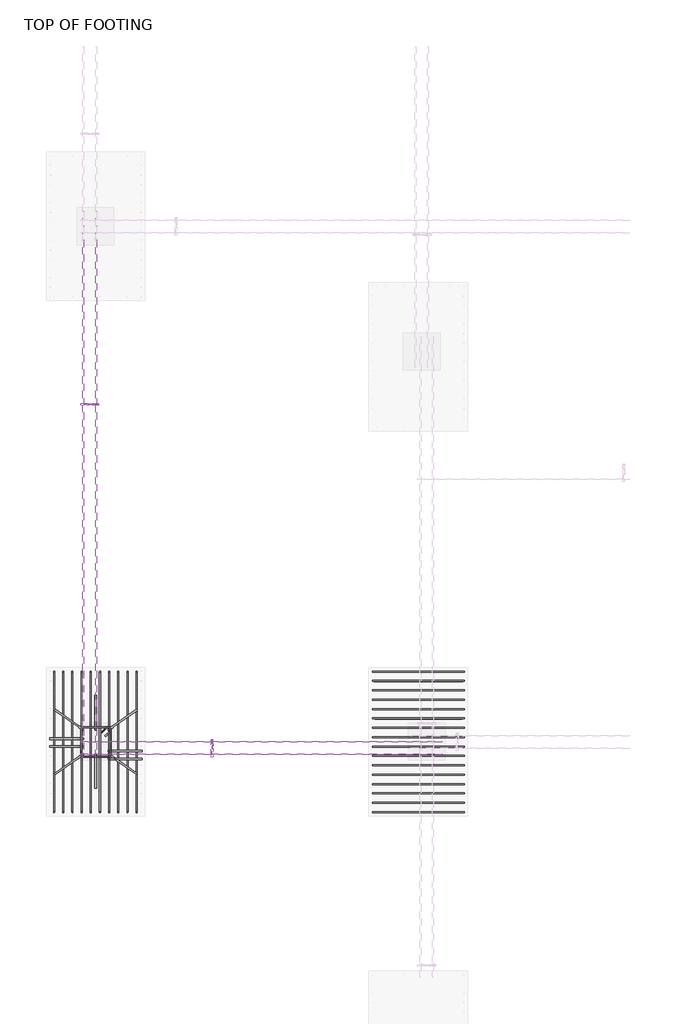
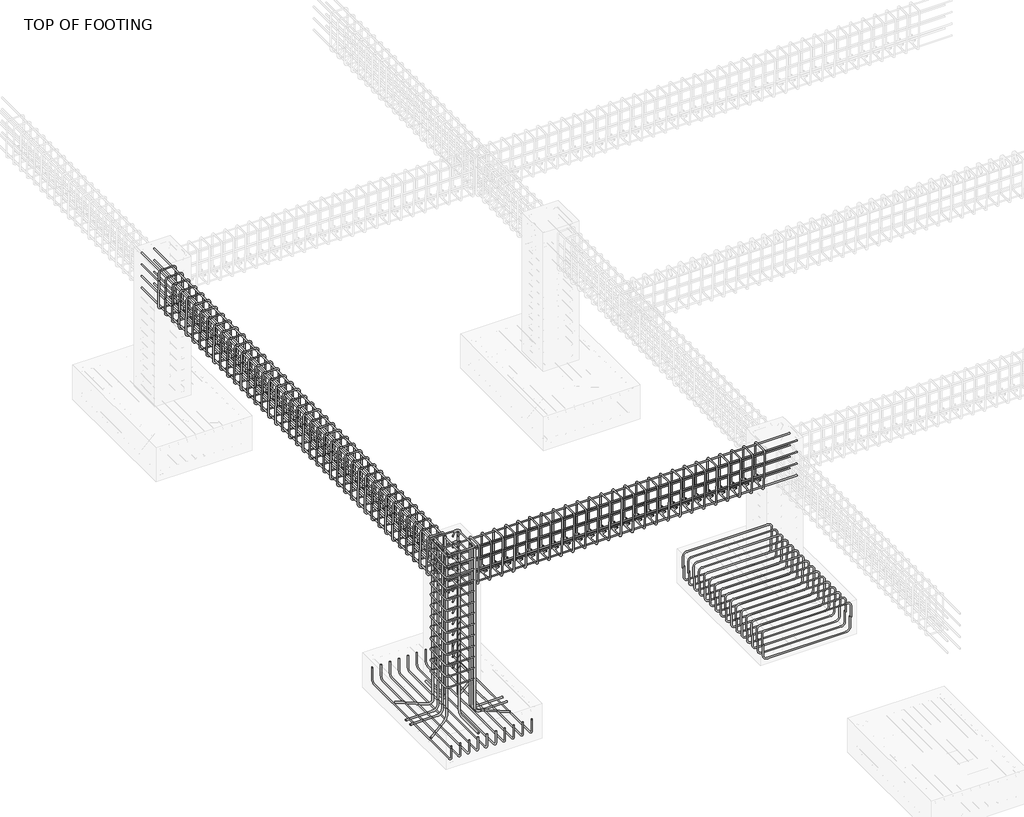
# One storey, part 3 of 11: 18 reinforcing bars.
"""IFC4 building model written with IfcOpenShell, lengths in millimetres."""

from ifc_helpers import new_model, si_unit, point, frame, origin, place, context, project, spatial, polyline, circle_curve, trimmed, segment, composite_curve, source, transform, mapped, element, save
from ifc_brep_helpers import swept_disk

model = new_model("IFC4")

# Units and contexts
model_context = context("Model", 3, world=origin())
ifc_project = project(units=[si_unit("LENGTHUNIT", "METRE", prefix="MILLI")], contexts=[model_context])

# Site, building, storey
site = spatial("IfcSite", under=ifc_project)
building = spatial("IfcBuilding", under=site)
storey = spatial("IfcBuildingStorey", under=building, Name="TOP OF FOOTING", Elevation=-1828.8)

# Reinforcing bars
placement = place(None, origin())
reinforcing_bar_shape = source(origin(), model_context, "Body", "SolidModel", [
    swept_disk(composite_curve([segment(polyline([(-6783.9053871, -2335.4013044, -2021.5298587), (-6783.9053871, -2335.4013044, -2168.8298587)]), True, "CONTINUOUS"), segment(trimmed(circle_curve(frame((-6783.9053871, -2381.7513044, -2168.8298587), z_axis=(-1.0, 0.0, 0.0), x_axis=(0.0, 46.350000000000364, 0.0)), 46.35), [point((-6783.9053871, -2335.4013044, -2168.8298587))], [point((-6783.9053871, -2381.7513044, -2215.1798587))], True, "CARTESIAN"), True, "CONTINUOUS"), segment(polyline([(-6783.9053871, -2381.7513044, -2215.1798587), (-6783.9053871, -3996.3513044, -2215.1798587)]), True, "CONTINUOUS"), segment(trimmed(circle_curve(frame((-6783.9053871, -3996.3513044, -2168.8298587), z_axis=(-1.0, 0.0, 0.0), x_axis=(0.0, 0.0, -46.34999999999991)), 46.35), [point((-6783.9053871, -3996.3513044, -2215.1798587))], [point((-6783.9053871, -4042.7013044, -2168.8298587))], True, "CARTESIAN"), True, "CONTINUOUS"), segment(polyline([(-6783.9053871, -4042.7013044, -2168.8298587), (-6783.9053871, -4042.7013044, -2021.5298587)]), True, "CONTINUOUS")], self_intersect=False), 6.35),
])
element("IfcReinforcingBar", 1, at=placement, inside=storey, context=model_context, shape_type="MappedRepresentation", body=[
    mapped(reinforcing_bar_shape, transform((0.0, 0.0, 0.0), x_axis=(1.0, 0.0, 0.0), y_axis=(0.0, 1.0, 0.0), z_axis=(0.0, 0.0, 1.0))),
    mapped(reinforcing_bar_shape, transform((111.55177, 0.0, 0.0), x_axis=(1.0, 0.0, 0.0), y_axis=(0.0, 1.0, 0.0), z_axis=(0.0, 0.0, 1.0))),
    mapped(reinforcing_bar_shape, transform((223.10354, 0.0, 0.0), x_axis=(1.0, 0.0, 0.0), y_axis=(0.0, 1.0, 0.0), z_axis=(0.0, 0.0, 1.0))),
    mapped(reinforcing_bar_shape, transform((334.6553099, 0.0, 0.0), x_axis=(1.0, 0.0, 0.0), y_axis=(0.0, 1.0, 0.0), z_axis=(0.0, 0.0, 1.0))),
    mapped(reinforcing_bar_shape, transform((446.2070799, 0.0, 0.0), x_axis=(1.0, 0.0, 0.0), y_axis=(0.0, 1.0, 0.0), z_axis=(0.0, 0.0, 1.0))),
    mapped(reinforcing_bar_shape, transform((557.7588499, 0.0, 0.0), x_axis=(1.0, 0.0, 0.0), y_axis=(0.0, 1.0, 0.0), z_axis=(0.0, 0.0, 1.0))),
    mapped(reinforcing_bar_shape, transform((669.3106199, 0.0, 0.0), x_axis=(1.0, 0.0, 0.0), y_axis=(0.0, 1.0, 0.0), z_axis=(0.0, 0.0, 1.0))),
    mapped(reinforcing_bar_shape, transform((780.8623899, 0.0, 0.0), x_axis=(1.0, 0.0, 0.0), y_axis=(0.0, 1.0, 0.0), z_axis=(0.0, 0.0, 1.0))),
    mapped(reinforcing_bar_shape, transform((892.4141599, 0.0, 0.0), x_axis=(1.0, 0.0, 0.0), y_axis=(0.0, 1.0, 0.0), z_axis=(0.0, 0.0, 1.0))),
    mapped(reinforcing_bar_shape, transform((1003.9659298, 0.0, 0.0), x_axis=(1.0, 0.0, 0.0), y_axis=(0.0, 1.0, 0.0), z_axis=(0.0, 0.0, 1.0))),
])
reinforcing_bar_2_shape = source(origin(), model_context, "Body", "SolidModel", [
    swept_disk(composite_curve([segment(polyline([(-1813.2210247, -2335.4013044, -2046.7466921), (-1813.2210247, -2335.4013044, -2194.0466921)]), True, "CONTINUOUS"), segment(trimmed(circle_curve(frame((-1859.5710247, -2335.4013044, -2194.0466921), z_axis=(0.0, 1.0, 0.0), x_axis=(46.34999999999991, 0.0, 0.0)), 46.35), [point((-1813.2210247, -2335.4013044, -2194.0466921))], [point((-1859.5710247, -2335.4013044, -2240.3966921))], True, "CARTESIAN"), True, "CONTINUOUS"), segment(polyline([(-1859.5710247, -2335.4013044, -2240.3966921), (-2850.7992774, -2335.4013044, -2240.3966921)]), True, "CONTINUOUS"), segment(trimmed(circle_curve(frame((-2850.7992774, -2335.4013044, -2194.0466921), z_axis=(0.0, 1.0, 0.0), x_axis=(0.0, 0.0, -46.34999999999991)), 46.35), [point((-2850.7992774, -2335.4013044, -2240.3966921))], [point((-2897.1492774, -2335.4013044, -2194.0466921))], True, "CARTESIAN"), True, "CONTINUOUS"), segment(polyline([(-2897.1492774, -2335.4013044, -2194.0466921), (-2897.1492774, -2335.4013044, -2046.7466921)]), True, "CONTINUOUS")], self_intersect=False), 6.35),
])
element("IfcReinforcingBar", 2, at=placement, inside=storey, context=model_context, shape_type="MappedRepresentation", body=[
    mapped(reinforcing_bar_2_shape, transform((0.0, 0.0, 0.0), x_axis=(1.0, 0.0, 0.0), y_axis=(0.0, 1.0, 0.0), z_axis=(0.0, 0.0, 1.0))),
    mapped(reinforcing_bar_2_shape, transform((0.0, -113.82, 0.0), x_axis=(1.0, 0.0, 0.0), y_axis=(0.0, 1.0, 0.0), z_axis=(0.0, 0.0, 1.0))),
    mapped(reinforcing_bar_2_shape, transform((0.0, -227.64, 0.0), x_axis=(1.0, 0.0, 0.0), y_axis=(0.0, 1.0, 0.0), z_axis=(0.0, 0.0, 1.0))),
    mapped(reinforcing_bar_2_shape, transform((0.0, -341.46, 0.0), x_axis=(1.0, 0.0, 0.0), y_axis=(0.0, 1.0, 0.0), z_axis=(0.0, 0.0, 1.0))),
    mapped(reinforcing_bar_2_shape, transform((0.0, -455.28, 0.0), x_axis=(1.0, 0.0, 0.0), y_axis=(0.0, 1.0, 0.0), z_axis=(0.0, 0.0, 1.0))),
    mapped(reinforcing_bar_2_shape, transform((0.0, -569.1, 0.0), x_axis=(1.0, 0.0, 0.0), y_axis=(0.0, 1.0, 0.0), z_axis=(0.0, 0.0, 1.0))),
    mapped(reinforcing_bar_2_shape, transform((0.0, -682.92, 0.0), x_axis=(1.0, 0.0, 0.0), y_axis=(0.0, 1.0, 0.0), z_axis=(0.0, 0.0, 1.0))),
    mapped(reinforcing_bar_2_shape, transform((0.0, -796.74, 0.0), x_axis=(1.0, 0.0, 0.0), y_axis=(0.0, 1.0, 0.0), z_axis=(0.0, 0.0, 1.0))),
    mapped(reinforcing_bar_2_shape, transform((0.0, -910.56, 0.0), x_axis=(1.0, 0.0, 0.0), y_axis=(0.0, 1.0, 0.0), z_axis=(0.0, 0.0, 1.0))),
    mapped(reinforcing_bar_2_shape, transform((0.0, -1024.38, 0.0), x_axis=(1.0, 0.0, 0.0), y_axis=(0.0, 1.0, 0.0), z_axis=(0.0, 0.0, 1.0))),
    mapped(reinforcing_bar_2_shape, transform((0.0, -1138.2, 0.0), x_axis=(1.0, 0.0, 0.0), y_axis=(0.0, 1.0, 0.0), z_axis=(0.0, 0.0, 1.0))),
    mapped(reinforcing_bar_2_shape, transform((0.0, -1252.02, 0.0), x_axis=(1.0, 0.0, 0.0), y_axis=(0.0, 1.0, 0.0), z_axis=(0.0, 0.0, 1.0))),
    mapped(reinforcing_bar_2_shape, transform((0.0, -1365.84, 0.0), x_axis=(1.0, 0.0, 0.0), y_axis=(0.0, 1.0, 0.0), z_axis=(0.0, 0.0, 1.0))),
    mapped(reinforcing_bar_2_shape, transform((0.0, -1479.66, 0.0), x_axis=(1.0, 0.0, 0.0), y_axis=(0.0, 1.0, 0.0), z_axis=(0.0, 0.0, 1.0))),
    mapped(reinforcing_bar_2_shape, transform((0.0, -1593.48, 0.0), x_axis=(1.0, 0.0, 0.0), y_axis=(0.0, 1.0, 0.0), z_axis=(0.0, 0.0, 1.0))),
    mapped(reinforcing_bar_2_shape, transform((0.0, -1707.3, 0.0), x_axis=(1.0, 0.0, 0.0), y_axis=(0.0, 1.0, 0.0), z_axis=(0.0, 0.0, 1.0))),
])
reinforcing_bar_3_shape = source(origin(), model_context, "Body", "SolidModel", [
    swept_disk(composite_curve([segment(polyline([(-2909.0228049, -2335.4013044, -2061.9958198), (-2909.0228049, -2335.4013044, -1914.6958198)]), True, "CONTINUOUS"), segment(trimmed(circle_curve(frame((-2862.6728049, -2335.4013044, -1914.6958198), z_axis=(0.0, 1.0, 0.0), x_axis=(-46.350000000000364, 0.0, 0.0)), 46.35), [point((-2909.0228049, -2335.4013044, -1914.6958198))], [point((-2862.6728049, -2335.4013044, -1868.3458198))], True, "CARTESIAN"), True, "CONTINUOUS"), segment(polyline([(-2862.6728049, -2335.4013044, -1868.3458198), (-1848.0728049, -2335.4013044, -1868.3458198)]), True, "CONTINUOUS"), segment(trimmed(circle_curve(frame((-1848.0728049, -2335.4013044, -1914.6958198), z_axis=(0.0, 1.0, 0.0), x_axis=(0.0, 0.0, 46.34999999999991)), 46.35), [point((-1848.0728049, -2335.4013044, -1868.3458198))], [point((-1801.7228049, -2335.4013044, -1914.6958198))], True, "CARTESIAN"), True, "CONTINUOUS"), segment(polyline([(-1801.7228049, -2335.4013044, -1914.6958198), (-1801.7228049, -2335.4013044, -2061.9958198)]), True, "CONTINUOUS")], self_intersect=False), 6.35),
])
element("IfcReinforcingBar", 3, at=placement, inside=storey, context=model_context, shape_type="MappedRepresentation", body=[
    mapped(reinforcing_bar_3_shape, transform((0.0, 0.0, 0.0), x_axis=(1.0, 0.0, 0.0), y_axis=(0.0, 1.0, 0.0), z_axis=(0.0, 0.0, 1.0))),
    mapped(reinforcing_bar_3_shape, transform((0.0, -113.82, 0.0), x_axis=(1.0, 0.0, 0.0), y_axis=(0.0, 1.0, 0.0), z_axis=(0.0, 0.0, 1.0))),
    mapped(reinforcing_bar_3_shape, transform((0.0, -227.64, 0.0), x_axis=(1.0, 0.0, 0.0), y_axis=(0.0, 1.0, 0.0), z_axis=(0.0, 0.0, 1.0))),
    mapped(reinforcing_bar_3_shape, transform((0.0, -341.46, 0.0), x_axis=(1.0, 0.0, 0.0), y_axis=(0.0, 1.0, 0.0), z_axis=(0.0, 0.0, 1.0))),
    mapped(reinforcing_bar_3_shape, transform((0.0, -455.28, 0.0), x_axis=(1.0, 0.0, 0.0), y_axis=(0.0, 1.0, 0.0), z_axis=(0.0, 0.0, 1.0))),
    mapped(reinforcing_bar_3_shape, transform((0.0, -569.1, 0.0), x_axis=(1.0, 0.0, 0.0), y_axis=(0.0, 1.0, 0.0), z_axis=(0.0, 0.0, 1.0))),
    mapped(reinforcing_bar_3_shape, transform((0.0, -682.92, 0.0), x_axis=(1.0, 0.0, 0.0), y_axis=(0.0, 1.0, 0.0), z_axis=(0.0, 0.0, 1.0))),
    mapped(reinforcing_bar_3_shape, transform((0.0, -796.74, 0.0), x_axis=(1.0, 0.0, 0.0), y_axis=(0.0, 1.0, 0.0), z_axis=(0.0, 0.0, 1.0))),
    mapped(reinforcing_bar_3_shape, transform((0.0, -910.56, 0.0), x_axis=(1.0, 0.0, 0.0), y_axis=(0.0, 1.0, 0.0), z_axis=(0.0, 0.0, 1.0))),
    mapped(reinforcing_bar_3_shape, transform((0.0, -1024.38, 0.0), x_axis=(1.0, 0.0, 0.0), y_axis=(0.0, 1.0, 0.0), z_axis=(0.0, 0.0, 1.0))),
    mapped(reinforcing_bar_3_shape, transform((0.0, -1138.2, 0.0), x_axis=(1.0, 0.0, 0.0), y_axis=(0.0, 1.0, 0.0), z_axis=(0.0, 0.0, 1.0))),
    mapped(reinforcing_bar_3_shape, transform((0.0, -1252.02, 0.0), x_axis=(1.0, 0.0, 0.0), y_axis=(0.0, 1.0, 0.0), z_axis=(0.0, 0.0, 1.0))),
    mapped(reinforcing_bar_3_shape, transform((0.0, -1365.84, 0.0), x_axis=(1.0, 0.0, 0.0), y_axis=(0.0, 1.0, 0.0), z_axis=(0.0, 0.0, 1.0))),
    mapped(reinforcing_bar_3_shape, transform((0.0, -1479.66, 0.0), x_axis=(1.0, 0.0, 0.0), y_axis=(0.0, 1.0, 0.0), z_axis=(0.0, 0.0, 1.0))),
    mapped(reinforcing_bar_3_shape, transform((0.0, -1593.48, 0.0), x_axis=(1.0, 0.0, 0.0), y_axis=(0.0, 1.0, 0.0), z_axis=(0.0, 0.0, 1.0))),
    mapped(reinforcing_bar_3_shape, transform((0.0, -1707.3, 0.0), x_axis=(1.0, 0.0, 0.0), y_axis=(0.0, 1.0, 0.0), z_axis=(0.0, 0.0, 1.0))),
])
reinforcing_bar_4_shape = source(origin(), model_context, "Body", "SolidModel", [
    swept_disk(composite_curve([segment(polyline([(-6205.9841654, -3075.3270697, -46.35), (-6150.2406025, -3019.5835068, -46.35)]), True, "CONTINUOUS"), segment(trimmed(circle_curve(frame((-6128.0728049, -3041.7513044, -46.35), z_axis=(0.0, 0.0, -1.0), x_axis=(-22.167797600000085, 22.167797600000085, 0.0)), 31.35), [point((-6150.2406025, -3019.5835068, -46.35))], [point((-6096.7228049, -3041.7513044, -46.35))], True, "CARTESIAN"), True, "CONTINUOUS"), segment(polyline([(-6096.7228049, -3041.7513044, -46.35), (-6096.7228049, -3336.3513044, -46.35)]), True, "CONTINUOUS"), segment(trimmed(circle_curve(frame((-6128.0728049, -3336.3513044, -46.35), z_axis=(0.0, 0.0, -1.0), x_axis=(31.350000000000364, 0.0, 0.0)), 31.35), [point((-6096.7228049, -3336.3513044, -46.35))], [point((-6128.0728049, -3367.7013044, -46.35))], True, "CARTESIAN"), True, "CONTINUOUS"), segment(polyline([(-6128.0728049, -3367.7013044, -46.35), (-6422.6728049, -3367.7013044, -46.35)]), True, "CONTINUOUS"), segment(trimmed(circle_curve(frame((-6422.6728049, -3336.3710895, -45.2363875), z_axis=(0.0, 0.0355219283344819, -0.9993688971583016), x_axis=(0.0, -31.3302149000001, -1.1136125000000021)), 31.35), [point((-6422.6728049, -3367.7013044, -46.35))], [point((-6454.0228049, -3336.3710895, -45.2363875))], True, "CARTESIAN"), True, "CONTINUOUS"), segment(polyline([(-6454.0228049, -3336.3710895, -45.2363875), (-6454.0228049, -3041.7315193, -34.7636125)]), True, "CONTINUOUS"), segment(trimmed(circle_curve(frame((-6422.6728049, -3041.7315193, -34.7636125), z_axis=(0.0, 0.0355219283344819, -0.9993688971583016), x_axis=(-31.349999999999454, 0.0, 0.0)), 31.35), [point((-6454.0228049, -3041.7315193, -34.7636125))], [point((-6422.6728049, -3010.4013044, -33.65))], True, "CARTESIAN"), True, "CONTINUOUS"), segment(polyline([(-6422.6728049, -3010.4013044, -33.65), (-6128.0728049, -3010.4013044, -33.65)]), True, "CONTINUOUS"), segment(trimmed(circle_curve(frame((-6128.0728049, -3041.7513044, -33.65), z_axis=(0.0, 0.0, -1.0), x_axis=(0.0, 31.350000000000364, 0.0)), 31.35), [point((-6128.0728049, -3010.4013044, -33.65))], [point((-6105.9050073, -3063.919102, -33.65))], True, "CARTESIAN"), True, "CONTINUOUS"), segment(polyline([(-6105.9050073, -3063.919102, -33.65), (-6161.6485703, -3119.6626649, -33.65)]), True, "CONTINUOUS")], self_intersect=False), 6.35),
])
element("IfcReinforcingBar", 4, at=placement, inside=storey, context=model_context, shape_type="MappedRepresentation", body=[
    mapped(reinforcing_bar_4_shape, transform((0.0, 0.0, 0.0), x_axis=(1.0, 0.0, 0.0), y_axis=(0.0, 1.0, 0.0), z_axis=(0.0, 0.0, 1.0))),
    mapped(reinforcing_bar_4_shape, transform((0.0, 0.0, -144.675), x_axis=(1.0, 0.0, 0.0), y_axis=(0.0, 1.0, 0.0), z_axis=(0.0, 0.0, 1.0))),
    mapped(reinforcing_bar_4_shape, transform((0.0, 0.0, -289.35), x_axis=(1.0, 0.0, 0.0), y_axis=(0.0, 1.0, 0.0), z_axis=(0.0, 0.0, 1.0))),
    mapped(reinforcing_bar_4_shape, transform((0.0, 0.0, -434.025), x_axis=(1.0, 0.0, 0.0), y_axis=(0.0, 1.0, 0.0), z_axis=(0.0, 0.0, 1.0))),
    mapped(reinforcing_bar_4_shape, transform((0.0, 0.0, -578.7), x_axis=(1.0, 0.0, 0.0), y_axis=(0.0, 1.0, 0.0), z_axis=(0.0, 0.0, 1.0))),
    mapped(reinforcing_bar_4_shape, transform((0.0, 0.0, -723.375), x_axis=(1.0, 0.0, 0.0), y_axis=(0.0, 1.0, 0.0), z_axis=(0.0, 0.0, 1.0))),
    mapped(reinforcing_bar_4_shape, transform((0.0, 0.0, -868.05), x_axis=(1.0, 0.0, 0.0), y_axis=(0.0, 1.0, 0.0), z_axis=(0.0, 0.0, 1.0))),
    mapped(reinforcing_bar_4_shape, transform((0.0, 0.0, -1012.725), x_axis=(1.0, 0.0, 0.0), y_axis=(0.0, 1.0, 0.0), z_axis=(0.0, 0.0, 1.0))),
    mapped(reinforcing_bar_4_shape, transform((0.0, 0.0, -1157.4), x_axis=(1.0, 0.0, 0.0), y_axis=(0.0, 1.0, 0.0), z_axis=(0.0, 0.0, 1.0))),
    mapped(reinforcing_bar_4_shape, transform((0.0, 0.0, -1302.075), x_axis=(1.0, 0.0, 0.0), y_axis=(0.0, 1.0, 0.0), z_axis=(0.0, 0.0, 1.0))),
    mapped(reinforcing_bar_4_shape, transform((0.0, 0.0, -1446.75), x_axis=(1.0, 0.0, 0.0), y_axis=(0.0, 1.0, 0.0), z_axis=(0.0, 0.0, 1.0))),
    mapped(reinforcing_bar_4_shape, transform((0.0, 0.0, -1591.425), x_axis=(1.0, 0.0, 0.0), y_axis=(0.0, 1.0, 0.0), z_axis=(0.0, 0.0, 1.0))),
    mapped(reinforcing_bar_4_shape, transform((0.0, 0.0, -1736.1), x_axis=(1.0, 0.0, 0.0), y_axis=(0.0, 1.0, 0.0), z_axis=(0.0, 0.0, 1.0))),
])
reinforcing_bar_5_shape = source(origin(), model_context, "Body", "SolidModel", [
    swept_disk(composite_curve([segment(polyline([(-6118.0728049, -3300.4586931, -40.0), (-6118.0728049, -3300.4586931, -2136.75)]), True, "CONTINUOUS"), segment(trimmed(circle_curve(frame((-6051.0228049, -3300.4586931, -2136.75), z_axis=(0.0, -1.0, 0.0), x_axis=(-67.05000000000018, 0.0, 0.0)), 67.05), [point((-6118.0728049, -3300.4586931, -2136.75))], [point((-6051.0228049, -3300.4586931, -2203.8))], True, "CARTESIAN"), True, "CONTINUOUS"), segment(polyline([(-6051.0228049, -3300.4586931, -2203.8), (-5715.3728049, -3300.4586931, -2203.8)]), True, "CONTINUOUS")], self_intersect=False), 9.55),
])
element("IfcReinforcingBar", 5, at=placement, inside=storey, context=model_context, shape_type="MappedRepresentation", body=[
    mapped(reinforcing_bar_5_shape, transform((0.0, 0.0, 0.0), x_axis=(1.0, 0.0, 0.0), y_axis=(0.0, 1.0, 0.0), z_axis=(0.0, 0.0, 1.0))),
    mapped(reinforcing_bar_5_shape, transform((0.0, -94.3634327, 0.0), x_axis=(1.0, 0.0, 0.0), y_axis=(0.0, 1.0, 0.0), z_axis=(0.0, 0.0, 1.0))),
])
element("IfcReinforcingBar", 6, at=placement, inside=storey, context=model_context, shape_type="SolidModel", body=[
    swept_disk(composite_curve([segment(polyline([(-6118.0728049, -3340.0013044, -40.0), (-6118.0728049, -3340.0013044, -2136.75)]), True, "CONTINUOUS"), segment(trimmed(circle_curve(frame((-6063.1486603, -3378.4596044, -2136.75), z_axis=(-0.5735764363510477, -0.8191520442889907, 0.0), x_axis=(-54.924144599999636, 38.45829999999978, 0.0)), 67.05), [point((-6118.0728049, -3340.0013044, -2136.75))], [point((-6063.1486603, -3378.4596044, -2203.8))], True, "CARTESIAN"), True, "CONTINUOUS"), segment(polyline([(-6063.1486603, -3378.4596044, -2203.8), (-5780.0087562, -3576.7162997, -2203.8)]), True, "CONTINUOUS")], self_intersect=False), 9.55),
])
element("IfcReinforcingBar", 7, at=placement, inside=storey, context=model_context, shape_type="SolidModel", body=[
    swept_disk(composite_curve([segment(polyline([(-6118.0728049, -3038.1013044, -40.0), (-6118.0728049, -3038.1013044, -2136.75)]), True, "CONTINUOUS"), segment(trimmed(circle_curve(frame((-6063.1486603, -2999.6430043, -2136.75), z_axis=(0.5735764363510477, -0.8191520442889908, 0.0), x_axis=(-54.924144599999636, -38.45830010000009, 0.0)), 67.05), [point((-6118.0728049, -3038.1013044, -2136.75))], [point((-6063.1486603, -2999.6430043, -2203.8))], True, "CARTESIAN"), True, "CONTINUOUS"), segment(polyline([(-6063.1486603, -2999.6430043, -2203.8), (-5780.0087562, -2801.3863091, -2203.8)]), True, "CONTINUOUS")], self_intersect=False), 9.55),
])
element("IfcReinforcingBar", 8, at=placement, inside=storey, context=model_context, shape_type="SolidModel", body=[
    swept_disk(composite_curve([segment(polyline([(-6432.6728049, -3340.0013044, -40.0), (-6432.6728049, -3340.0013044, -2136.75)]), True, "CONTINUOUS"), segment(trimmed(circle_curve(frame((-6487.5969495, -3378.4596044, -2136.75), z_axis=(-0.5735764363510477, 0.8191520442889908, 0.0), x_axis=(54.924144599999636, 38.45829999999978, 0.0)), 67.05), [point((-6432.6728049, -3340.0013044, -2136.75))], [point((-6487.5969495, -3378.4596044, -2203.8))], True, "CARTESIAN"), True, "CONTINUOUS"), segment(polyline([(-6487.5969495, -3378.4596044, -2203.8), (-6770.7368536, -3576.7162997, -2203.8)]), True, "CONTINUOUS")], self_intersect=False), 9.55),
])
element("IfcReinforcingBar", 9, at=placement, inside=storey, context=model_context, shape_type="SolidModel", body=[
    swept_disk(composite_curve([segment(polyline([(-6432.6728049, -3038.1013044, -40.0), (-6432.6728049, -3038.1013044, -2136.75)]), True, "CONTINUOUS"), segment(trimmed(circle_curve(frame((-6487.5969495, -2999.6430043, -2136.75), z_axis=(0.5735764363510477, 0.8191520442889907, 0.0), x_axis=(54.924144599999636, -38.45830010000009, 0.0)), 67.05), [point((-6432.6728049, -3038.1013044, -2136.75))], [point((-6487.5969495, -2999.6430043, -2203.8))], True, "CARTESIAN"), True, "CONTINUOUS"), segment(polyline([(-6487.5969495, -2999.6430043, -2203.8), (-6770.7368536, -2801.3863091, -2203.8)]), True, "CONTINUOUS")], self_intersect=False), 9.55),
])
reinforcing_bar_6_shape = source(origin(), model_context, "Body", "SolidModel", [
    swept_disk(composite_curve([segment(polyline([(-6432.6728049, -3150.4586931, -40.0), (-6432.6728049, -3150.4586931, -2136.75)]), True, "CONTINUOUS"), segment(trimmed(circle_curve(frame((-6499.7228049, -3150.4586931, -2136.75), z_axis=(0.0, 1.0, 0.0), x_axis=(67.04999999999927, 0.0, 0.0)), 67.05), [point((-6432.6728049, -3150.4586931, -2136.75))], [point((-6499.7228049, -3150.4586931, -2203.8))], True, "CARTESIAN"), True, "CONTINUOUS"), segment(polyline([(-6499.7228049, -3150.4586931, -2203.8), (-6835.3728049, -3150.4586931, -2203.8)]), True, "CONTINUOUS")], self_intersect=False), 9.55),
])
element("IfcReinforcingBar", 10, at=placement, inside=storey, context=model_context, shape_type="MappedRepresentation", body=[
    mapped(reinforcing_bar_6_shape, transform((0.0, 0.0, 0.0), x_axis=(1.0, 0.0, 0.0), y_axis=(0.0, 1.0, 0.0), z_axis=(0.0, 0.0, 1.0))),
    mapped(reinforcing_bar_6_shape, transform((0.0, -94.3634327, 0.0), x_axis=(1.0, 0.0, 0.0), y_axis=(0.0, 1.0, 0.0), z_axis=(0.0, 0.0, 1.0))),
])
element("IfcReinforcingBar", 11, at=placement, inside=storey, context=model_context, shape_type="SolidModel", body=[
    swept_disk(composite_curve([segment(polyline([(-6278.0728049, -3038.1013044, -40.0), (-6278.0728049, -3038.1013044, -2136.75)]), True, "CONTINUOUS"), segment(trimmed(circle_curve(frame((-6278.0728049, -2971.0513044, -2136.75), z_axis=(1.0, 0.0, 0.0), x_axis=(0.0, -67.05000000000018, 0.0)), 67.05), [point((-6278.0728049, -3038.1013044, -2136.75))], [point((-6278.0728049, -2971.0513044, -2203.8))], True, "CARTESIAN"), True, "CONTINUOUS"), segment(polyline([(-6278.0728049, -2971.0513044, -2203.8), (-6278.0728049, -2625.4013044, -2203.8)]), True, "CONTINUOUS")], self_intersect=False), 9.55),
])
element("IfcReinforcingBar", 12, at=placement, inside=storey, context=model_context, shape_type="SolidModel", body=[
    swept_disk(composite_curve([segment(polyline([(-6278.0728049, -3340.0013044, -40.0), (-6278.0728049, -3340.0013044, -2136.75)]), True, "CONTINUOUS"), segment(trimmed(circle_curve(frame((-6278.0728049, -3407.0513044, -2136.75), z_axis=(-1.0, 0.0, 0.0), x_axis=(0.0, 67.04999999999973, 0.0)), 67.05), [point((-6278.0728049, -3340.0013044, -2136.75))], [point((-6278.0728049, -3407.0513044, -2203.8))], True, "CARTESIAN"), True, "CONTINUOUS"), segment(polyline([(-6278.0728049, -3407.0513044, -2203.8), (-6278.0728049, -3752.7013044, -2203.8)]), True, "CONTINUOUS")], self_intersect=False), 9.55),
])
reinforcing_bar_7_shape = source(origin(), model_context, "Body", "SolidModel", [
    swept_disk(composite_curve([segment(polyline([(-6355.9841654, 2837.5044674, -488.7242346), (-6300.2406025, 2837.5044674, -544.4677976)]), True, "CONTINUOUS"), segment(trimmed(circle_curve(frame((-6278.0728049, 2837.5044674, -522.3), z_axis=(0.0, -1.0, 0.0), x_axis=(-22.167797600000085, 0.0, -22.167797600000085)), 31.35), [point((-6300.2406025, 2837.5044674, -544.4677976))], [point((-6246.7228049, 2837.5044674, -522.3))], True, "CARTESIAN"), True, "CONTINUOUS"), segment(polyline([(-6246.7228049, 2837.5044674, -522.3), (-6246.7228049, 2837.5044674, -77.7)]), True, "CONTINUOUS"), segment(trimmed(circle_curve(frame((-6278.0728049, 2837.5044674, -77.7), z_axis=(0.0, -1.0, 0.0), x_axis=(31.350000000000364, 0.0, 0.0)), 31.35), [point((-6246.7228049, 2837.5044674, -77.7))], [point((-6278.0728049, 2837.5044674, -46.35))], True, "CARTESIAN"), True, "CONTINUOUS"), segment(polyline([(-6278.0728049, 2837.5044674, -46.35), (-6422.6728049, 2837.5044674, -46.35)]), True, "CONTINUOUS"), segment(trimmed(circle_curve(frame((-6422.6728049, 2838.289053, -77.6901807), z_axis=(0.0, -0.9996867842138424, -0.025026655153786322), x_axis=(0.0, -0.7845855999999003, 31.340180699999998)), 31.35), [point((-6422.6728049, 2837.5044674, -46.35))], [point((-6454.0228049, 2838.289053, -77.6901807))], True, "CARTESIAN"), True, "CONTINUOUS"), segment(polyline([(-6454.0228049, 2838.289053, -77.6901807), (-6454.0228049, 2849.4198817, -522.3098193)]), True, "CONTINUOUS"), segment(trimmed(circle_curve(frame((-6422.6728049, 2849.4198817, -522.3098193), z_axis=(0.0, -0.9996867842138424, -0.025026655153786322), x_axis=(-31.349999999999454, 0.0, 0.0)), 31.35), [point((-6454.0228049, 2849.4198817, -522.3098193))], [point((-6422.6728049, 2850.2044674, -553.65))], True, "CARTESIAN"), True, "CONTINUOUS"), segment(polyline([(-6422.6728049, 2850.2044674, -553.65), (-6278.0728049, 2850.2044674, -553.65)]), True, "CONTINUOUS"), segment(trimmed(circle_curve(frame((-6278.0728049, 2850.2044674, -522.3), z_axis=(0.0, -1.0, 0.0), x_axis=(0.0, 0.0, -31.350000000000023)), 31.35), [point((-6278.0728049, 2850.2044674, -553.65))], [point((-6255.9050073, 2850.2044674, -500.1322024))], True, "CARTESIAN"), True, "CONTINUOUS"), segment(polyline([(-6255.9050073, 2850.2044674, -500.1322024), (-6311.6485703, 2850.2044674, -444.3886395)]), True, "CONTINUOUS")], self_intersect=False), 6.35),
])
element("IfcReinforcingBar", 13, at=placement, inside=storey, context=model_context, shape_type="MappedRepresentation", body=[
    mapped(reinforcing_bar_7_shape, transform((0.0, 0.0, 0.0), x_axis=(1.0, 0.0, 0.0), y_axis=(0.0, 1.0, 0.0), z_axis=(0.0, 0.0, 1.0))),
    mapped(reinforcing_bar_7_shape, transform((0.0, -148.5950198, 0.0), x_axis=(1.0, 0.0, 0.0), y_axis=(0.0, 1.0, 0.0), z_axis=(0.0, 0.0, 1.0))),
    mapped(reinforcing_bar_7_shape, transform((0.0, -297.1900396, 0.0), x_axis=(1.0, 0.0, 0.0), y_axis=(0.0, 1.0, 0.0), z_axis=(0.0, 0.0, 1.0))),
    mapped(reinforcing_bar_7_shape, transform((0.0, -445.7850594, 0.0), x_axis=(1.0, 0.0, 0.0), y_axis=(0.0, 1.0, 0.0), z_axis=(0.0, 0.0, 1.0))),
    mapped(reinforcing_bar_7_shape, transform((0.0, -594.3800792, 0.0), x_axis=(1.0, 0.0, 0.0), y_axis=(0.0, 1.0, 0.0), z_axis=(0.0, 0.0, 1.0))),
    mapped(reinforcing_bar_7_shape, transform((0.0, -742.9750989, 0.0), x_axis=(1.0, 0.0, 0.0), y_axis=(0.0, 1.0, 0.0), z_axis=(0.0, 0.0, 1.0))),
    mapped(reinforcing_bar_7_shape, transform((0.0, -891.5701187, 0.0), x_axis=(1.0, 0.0, 0.0), y_axis=(0.0, 1.0, 0.0), z_axis=(0.0, 0.0, 1.0))),
    mapped(reinforcing_bar_7_shape, transform((0.0, -1040.1651385, 0.0), x_axis=(1.0, 0.0, 0.0), y_axis=(0.0, 1.0, 0.0), z_axis=(0.0, 0.0, 1.0))),
    mapped(reinforcing_bar_7_shape, transform((0.0, -1188.7601583, 0.0), x_axis=(1.0, 0.0, 0.0), y_axis=(0.0, 1.0, 0.0), z_axis=(0.0, 0.0, 1.0))),
    mapped(reinforcing_bar_7_shape, transform((0.0, -1337.3551781, 0.0), x_axis=(1.0, 0.0, 0.0), y_axis=(0.0, 1.0, 0.0), z_axis=(0.0, 0.0, 1.0))),
    mapped(reinforcing_bar_7_shape, transform((0.0, -1485.9501979, 0.0), x_axis=(1.0, 0.0, 0.0), y_axis=(0.0, 1.0, 0.0), z_axis=(0.0, 0.0, 1.0))),
    mapped(reinforcing_bar_7_shape, transform((0.0, -1634.5452177, 0.0), x_axis=(1.0, 0.0, 0.0), y_axis=(0.0, 1.0, 0.0), z_axis=(0.0, 0.0, 1.0))),
    mapped(reinforcing_bar_7_shape, transform((0.0, -1783.1402375, 0.0), x_axis=(1.0, 0.0, 0.0), y_axis=(0.0, 1.0, 0.0), z_axis=(0.0, 0.0, 1.0))),
    mapped(reinforcing_bar_7_shape, transform((0.0, -1931.7352573, 0.0), x_axis=(1.0, 0.0, 0.0), y_axis=(0.0, 1.0, 0.0), z_axis=(0.0, 0.0, 1.0))),
    mapped(reinforcing_bar_7_shape, transform((0.0, -2080.330277, 0.0), x_axis=(1.0, 0.0, 0.0), y_axis=(0.0, 1.0, 0.0), z_axis=(0.0, 0.0, 1.0))),
    mapped(reinforcing_bar_7_shape, transform((0.0, -2228.9252968, 0.0), x_axis=(1.0, 0.0, 0.0), y_axis=(0.0, 1.0, 0.0), z_axis=(0.0, 0.0, 1.0))),
    mapped(reinforcing_bar_7_shape, transform((0.0, -2377.5203166, 0.0), x_axis=(1.0, 0.0, 0.0), y_axis=(0.0, 1.0, 0.0), z_axis=(0.0, 0.0, 1.0))),
    mapped(reinforcing_bar_7_shape, transform((0.0, -2526.1153364, 0.0), x_axis=(1.0, 0.0, 0.0), y_axis=(0.0, 1.0, 0.0), z_axis=(0.0, 0.0, 1.0))),
    mapped(reinforcing_bar_7_shape, transform((0.0, -2674.7103562, 0.0), x_axis=(1.0, 0.0, 0.0), y_axis=(0.0, 1.0, 0.0), z_axis=(0.0, 0.0, 1.0))),
    mapped(reinforcing_bar_7_shape, transform((0.0, -2823.305376, 0.0), x_axis=(1.0, 0.0, 0.0), y_axis=(0.0, 1.0, 0.0), z_axis=(0.0, 0.0, 1.0))),
    mapped(reinforcing_bar_7_shape, transform((0.0, -2971.9003958, 0.0), x_axis=(1.0, 0.0, 0.0), y_axis=(0.0, 1.0, 0.0), z_axis=(0.0, 0.0, 1.0))),
    mapped(reinforcing_bar_7_shape, transform((0.0, -3120.4954156, 0.0), x_axis=(1.0, 0.0, 0.0), y_axis=(0.0, 1.0, 0.0), z_axis=(0.0, 0.0, 1.0))),
    mapped(reinforcing_bar_7_shape, transform((0.0, -3269.0904354, 0.0), x_axis=(1.0, 0.0, 0.0), y_axis=(0.0, 1.0, 0.0), z_axis=(0.0, 0.0, 1.0))),
    mapped(reinforcing_bar_7_shape, transform((0.0, -3417.6854551, 0.0), x_axis=(1.0, 0.0, 0.0), y_axis=(0.0, 1.0, 0.0), z_axis=(0.0, 0.0, 1.0))),
    mapped(reinforcing_bar_7_shape, transform((0.0, -3566.2804749, 0.0), x_axis=(1.0, 0.0, 0.0), y_axis=(0.0, 1.0, 0.0), z_axis=(0.0, 0.0, 1.0))),
    mapped(reinforcing_bar_7_shape, transform((0.0, -3714.8754947, 0.0), x_axis=(1.0, 0.0, 0.0), y_axis=(0.0, 1.0, 0.0), z_axis=(0.0, 0.0, 1.0))),
    mapped(reinforcing_bar_7_shape, transform((0.0, -3863.4705145, 0.0), x_axis=(1.0, 0.0, 0.0), y_axis=(0.0, 1.0, 0.0), z_axis=(0.0, 0.0, 1.0))),
    mapped(reinforcing_bar_7_shape, transform((0.0, -4012.0655343, 0.0), x_axis=(1.0, 0.0, 0.0), y_axis=(0.0, 1.0, 0.0), z_axis=(0.0, 0.0, 1.0))),
    mapped(reinforcing_bar_7_shape, transform((0.0, -4160.6605541, 0.0), x_axis=(1.0, 0.0, 0.0), y_axis=(0.0, 1.0, 0.0), z_axis=(0.0, 0.0, 1.0))),
    mapped(reinforcing_bar_7_shape, transform((0.0, -4309.2555739, 0.0), x_axis=(1.0, 0.0, 0.0), y_axis=(0.0, 1.0, 0.0), z_axis=(0.0, 0.0, 1.0))),
    mapped(reinforcing_bar_7_shape, transform((0.0, -4457.8505937, 0.0), x_axis=(1.0, 0.0, 0.0), y_axis=(0.0, 1.0, 0.0), z_axis=(0.0, 0.0, 1.0))),
    mapped(reinforcing_bar_7_shape, transform((0.0, -4606.4456135, 0.0), x_axis=(1.0, 0.0, 0.0), y_axis=(0.0, 1.0, 0.0), z_axis=(0.0, 0.0, 1.0))),
    mapped(reinforcing_bar_7_shape, transform((0.0, -4755.0406332, 0.0), x_axis=(1.0, 0.0, 0.0), y_axis=(0.0, 1.0, 0.0), z_axis=(0.0, 0.0, 1.0))),
    mapped(reinforcing_bar_7_shape, transform((0.0, -4903.635653, 0.0), x_axis=(1.0, 0.0, 0.0), y_axis=(0.0, 1.0, 0.0), z_axis=(0.0, 0.0, 1.0))),
    mapped(reinforcing_bar_7_shape, transform((0.0, -5052.2306728, 0.0), x_axis=(1.0, 0.0, 0.0), y_axis=(0.0, 1.0, 0.0), z_axis=(0.0, 0.0, 1.0))),
    mapped(reinforcing_bar_7_shape, transform((0.0, -5200.8256926, 0.0), x_axis=(1.0, 0.0, 0.0), y_axis=(0.0, 1.0, 0.0), z_axis=(0.0, 0.0, 1.0))),
    mapped(reinforcing_bar_7_shape, transform((0.0, -5349.4207124, 0.0), x_axis=(1.0, 0.0, 0.0), y_axis=(0.0, 1.0, 0.0), z_axis=(0.0, 0.0, 1.0))),
    mapped(reinforcing_bar_7_shape, transform((0.0, -5498.0157322, 0.0), x_axis=(1.0, 0.0, 0.0), y_axis=(0.0, 1.0, 0.0), z_axis=(0.0, 0.0, 1.0))),
    mapped(reinforcing_bar_7_shape, transform((0.0, -5646.610752, 0.0), x_axis=(1.0, 0.0, 0.0), y_axis=(0.0, 1.0, 0.0), z_axis=(0.0, 0.0, 1.0))),
    mapped(reinforcing_bar_7_shape, transform((0.0, -5795.2057718, 0.0), x_axis=(1.0, 0.0, 0.0), y_axis=(0.0, 1.0, 0.0), z_axis=(0.0, 0.0, 1.0))),
])
reinforcing_bar_8_shape = source(origin(), model_context, "Body", "SolidModel", [
    swept_disk(composite_curve([segment(polyline([(-6273.0728049, 3253.8544674, -528.2977114), (-6273.0728049, -3374.0513044, -528.2977114)]), True, "CONTINUOUS")], self_intersect=False), 6.35),
])
element("IfcReinforcingBar", 14, at=placement, inside=storey, context=model_context, shape_type="MappedRepresentation", body=[
    mapped(reinforcing_bar_8_shape, transform((0.0, 0.0, 0.0), x_axis=(1.0, 0.0, 0.0), y_axis=(0.0, 1.0, 0.0), z_axis=(0.0, 0.0, 1.0))),
    mapped(reinforcing_bar_8_shape, transform((0.0, 0.0, 153.3723948), x_axis=(1.0, 0.0, 0.0), y_axis=(0.0, 1.0, 0.0), z_axis=(0.0, 0.0, 1.0))),
    mapped(reinforcing_bar_8_shape, transform((0.0, 0.0, 306.7447895), x_axis=(1.0, 0.0, 0.0), y_axis=(0.0, 1.0, 0.0), z_axis=(0.0, 0.0, 1.0))),
    mapped(reinforcing_bar_8_shape, transform((0.0, 0.0, 460.1171843), x_axis=(1.0, 0.0, 0.0), y_axis=(0.0, 1.0, 0.0), z_axis=(0.0, 0.0, 1.0))),
])
reinforcing_bar_9_shape = source(origin(), model_context, "Body", "SolidModel", [
    swept_disk(composite_curve([segment(polyline([(-6427.6728049, 3253.8544674, -528.2977114), (-6427.6728049, -3374.0513044, -528.2977114)]), True, "CONTINUOUS")], self_intersect=False), 6.35),
])
element("IfcReinforcingBar", 15, at=placement, inside=storey, context=model_context, shape_type="MappedRepresentation", body=[
    mapped(reinforcing_bar_9_shape, transform((0.0, 0.0, 0.0), x_axis=(1.0, 0.0, 0.0), y_axis=(0.0, 1.0, 0.0), z_axis=(0.0, 0.0, 1.0))),
    mapped(reinforcing_bar_9_shape, transform((0.0, 0.0, 153.3723948), x_axis=(1.0, 0.0, 0.0), y_axis=(0.0, 1.0, 0.0), z_axis=(0.0, 0.0, 1.0))),
    mapped(reinforcing_bar_9_shape, transform((0.0, 0.0, 306.7447895), x_axis=(1.0, 0.0, 0.0), y_axis=(0.0, 1.0, 0.0), z_axis=(0.0, 0.0, 1.0))),
    mapped(reinforcing_bar_9_shape, transform((0.0, 0.0, 460.1171843), x_axis=(1.0, 0.0, 0.0), y_axis=(0.0, 1.0, 0.0), z_axis=(0.0, 0.0, 1.0))),
])
reinforcing_bar_10_shape = source(origin(), model_context, "Body", "SolidModel", [
    swept_disk(composite_curve([segment(polyline([(-6044.0228049, -3269.6626649, -488.7242346), (-6044.0228049, -3213.919102, -544.4677976)]), True, "CONTINUOUS"), segment(trimmed(circle_curve(frame((-6044.0228049, -3191.7513044, -522.3), z_axis=(1.0, 0.0, 0.0), x_axis=(0.0, -22.16779759999963, -22.167797600000085)), 31.35), [point((-6044.0228049, -3213.919102, -544.4677976))], [point((-6044.0228049, -3160.4013044, -522.3))], True, "CARTESIAN"), True, "CONTINUOUS"), segment(polyline([(-6044.0228049, -3160.4013044, -522.3), (-6044.0228049, -3160.4013044, -77.7)]), True, "CONTINUOUS"), segment(trimmed(circle_curve(frame((-6044.0228049, -3191.7513044, -77.7), z_axis=(1.0, 0.0, 0.0), x_axis=(0.0, 31.350000000000364, 0.0)), 31.35), [point((-6044.0228049, -3160.4013044, -77.7))], [point((-6044.0228049, -3191.7513044, -46.35))], True, "CARTESIAN"), True, "CONTINUOUS"), segment(polyline([(-6044.0228049, -3191.7513044, -46.35), (-6044.0228049, -3336.3513044, -46.35)]), True, "CONTINUOUS"), segment(trimmed(circle_curve(frame((-6044.8073905, -3336.3513044, -77.6901807), z_axis=(0.9996867842138424, 0.0, -0.025026655153786322), x_axis=(0.784585600000355, 0.0, 31.340180699999998)), 31.35), [point((-6044.0228049, -3336.3513044, -46.35))], [point((-6044.8073905, -3367.7013044, -77.6901807))], True, "CARTESIAN"), True, "CONTINUOUS"), segment(polyline([(-6044.8073905, -3367.7013044, -77.6901807), (-6055.9382193, -3367.7013044, -522.3098193)]), True, "CONTINUOUS"), segment(trimmed(circle_curve(frame((-6055.9382193, -3336.3513044, -522.3098193), z_axis=(0.9996867842138424, 0.0, -0.025026655153786322), x_axis=(0.0, -31.34999999999991, 0.0)), 31.35), [point((-6055.9382193, -3367.7013044, -522.3098193))], [point((-6056.7228049, -3336.3513044, -553.65))], True, "CARTESIAN"), True, "CONTINUOUS"), segment(polyline([(-6056.7228049, -3336.3513044, -553.65), (-6056.7228049, -3191.7513044, -553.65)]), True, "CONTINUOUS"), segment(trimmed(circle_curve(frame((-6056.7228049, -3191.7513044, -522.3), z_axis=(1.0, 0.0, 0.0), x_axis=(0.0, 0.0, -31.350000000000023)), 31.35), [point((-6056.7228049, -3191.7513044, -553.65))], [point((-6056.7228049, -3169.5835068, -500.1322024))], True, "CARTESIAN"), True, "CONTINUOUS"), segment(polyline([(-6056.7228049, -3169.5835068, -500.1322024), (-6056.7228049, -3225.3270697, -444.3886395)]), True, "CONTINUOUS")], self_intersect=False), 6.35),
])
element("IfcReinforcingBar", 16, at=placement, inside=storey, context=model_context, shape_type="MappedRepresentation", body=[
    mapped(reinforcing_bar_10_shape, transform((0.0, 0.0, 0.0), x_axis=(1.0, 0.0, 0.0), y_axis=(0.0, 1.0, 0.0), z_axis=(0.0, 0.0, 1.0))),
    mapped(reinforcing_bar_10_shape, transform((148.2208333, 0.0, 0.0), x_axis=(1.0, 0.0, 0.0), y_axis=(0.0, 1.0, 0.0), z_axis=(0.0, 0.0, 1.0))),
    mapped(reinforcing_bar_10_shape, transform((296.4416667, 0.0, 0.0), x_axis=(1.0, 0.0, 0.0), y_axis=(0.0, 1.0, 0.0), z_axis=(0.0, 0.0, 1.0))),
    mapped(reinforcing_bar_10_shape, transform((444.6625, 0.0, 0.0), x_axis=(1.0, 0.0, 0.0), y_axis=(0.0, 1.0, 0.0), z_axis=(0.0, 0.0, 1.0))),
    mapped(reinforcing_bar_10_shape, transform((592.8833333, 0.0, 0.0), x_axis=(1.0, 0.0, 0.0), y_axis=(0.0, 1.0, 0.0), z_axis=(0.0, 0.0, 1.0))),
    mapped(reinforcing_bar_10_shape, transform((741.1041667, 0.0, 0.0), x_axis=(1.0, 0.0, 0.0), y_axis=(0.0, 1.0, 0.0), z_axis=(0.0, 0.0, 1.0))),
    mapped(reinforcing_bar_10_shape, transform((889.325, 0.0, 0.0), x_axis=(1.0, 0.0, 0.0), y_axis=(0.0, 1.0, 0.0), z_axis=(0.0, 0.0, 1.0))),
    mapped(reinforcing_bar_10_shape, transform((1037.5458333, 0.0, 0.0), x_axis=(1.0, 0.0, 0.0), y_axis=(0.0, 1.0, 0.0), z_axis=(0.0, 0.0, 1.0))),
    mapped(reinforcing_bar_10_shape, transform((1185.7666667, 0.0, 0.0), x_axis=(1.0, 0.0, 0.0), y_axis=(0.0, 1.0, 0.0), z_axis=(0.0, 0.0, 1.0))),
    mapped(reinforcing_bar_10_shape, transform((1333.9875, 0.0, 0.0), x_axis=(1.0, 0.0, 0.0), y_axis=(0.0, 1.0, 0.0), z_axis=(0.0, 0.0, 1.0))),
    mapped(reinforcing_bar_10_shape, transform((1482.2083333, 0.0, 0.0), x_axis=(1.0, 0.0, 0.0), y_axis=(0.0, 1.0, 0.0), z_axis=(0.0, 0.0, 1.0))),
    mapped(reinforcing_bar_10_shape, transform((1630.4291667, 0.0, 0.0), x_axis=(1.0, 0.0, 0.0), y_axis=(0.0, 1.0, 0.0), z_axis=(0.0, 0.0, 1.0))),
    mapped(reinforcing_bar_10_shape, transform((1778.65, 0.0, 0.0), x_axis=(1.0, 0.0, 0.0), y_axis=(0.0, 1.0, 0.0), z_axis=(0.0, 0.0, 1.0))),
    mapped(reinforcing_bar_10_shape, transform((1926.8708333, 0.0, 0.0), x_axis=(1.0, 0.0, 0.0), y_axis=(0.0, 1.0, 0.0), z_axis=(0.0, 0.0, 1.0))),
    mapped(reinforcing_bar_10_shape, transform((2075.0916667, 0.0, 0.0), x_axis=(1.0, 0.0, 0.0), y_axis=(0.0, 1.0, 0.0), z_axis=(0.0, 0.0, 1.0))),
    mapped(reinforcing_bar_10_shape, transform((2223.3125, 0.0, 0.0), x_axis=(1.0, 0.0, 0.0), y_axis=(0.0, 1.0, 0.0), z_axis=(0.0, 0.0, 1.0))),
    mapped(reinforcing_bar_10_shape, transform((2371.5333333, 0.0, 0.0), x_axis=(1.0, 0.0, 0.0), y_axis=(0.0, 1.0, 0.0), z_axis=(0.0, 0.0, 1.0))),
    mapped(reinforcing_bar_10_shape, transform((2519.7541667, 0.0, 0.0), x_axis=(1.0, 0.0, 0.0), y_axis=(0.0, 1.0, 0.0), z_axis=(0.0, 0.0, 1.0))),
    mapped(reinforcing_bar_10_shape, transform((2667.975, 0.0, 0.0), x_axis=(1.0, 0.0, 0.0), y_axis=(0.0, 1.0, 0.0), z_axis=(0.0, 0.0, 1.0))),
    mapped(reinforcing_bar_10_shape, transform((2816.1958333, 0.0, 0.0), x_axis=(1.0, 0.0, 0.0), y_axis=(0.0, 1.0, 0.0), z_axis=(0.0, 0.0, 1.0))),
    mapped(reinforcing_bar_10_shape, transform((2964.4166667, 0.0, 0.0), x_axis=(1.0, 0.0, 0.0), y_axis=(0.0, 1.0, 0.0), z_axis=(0.0, 0.0, 1.0))),
    mapped(reinforcing_bar_10_shape, transform((3112.6375, 0.0, 0.0), x_axis=(1.0, 0.0, 0.0), y_axis=(0.0, 1.0, 0.0), z_axis=(0.0, 0.0, 1.0))),
    mapped(reinforcing_bar_10_shape, transform((3260.8583333, 0.0, 0.0), x_axis=(1.0, 0.0, 0.0), y_axis=(0.0, 1.0, 0.0), z_axis=(0.0, 0.0, 1.0))),
    mapped(reinforcing_bar_10_shape, transform((3409.0791667, 0.0, 0.0), x_axis=(1.0, 0.0, 0.0), y_axis=(0.0, 1.0, 0.0), z_axis=(0.0, 0.0, 1.0))),
    mapped(reinforcing_bar_10_shape, transform((3557.3, 0.0, 0.0), x_axis=(1.0, 0.0, 0.0), y_axis=(0.0, 1.0, 0.0), z_axis=(0.0, 0.0, 1.0))),
])
reinforcing_bar_11_shape = source(origin(), model_context, "Body", "SolidModel", [
    swept_disk(composite_curve([segment(polyline([(-6460.3728049, -3186.7513044, -528.2977114), (-2070.3728049, -3186.7513044, -528.2977114)]), True, "CONTINUOUS")], self_intersect=False), 6.35),
])
element("IfcReinforcingBar", 17, at=placement, inside=storey, context=model_context, shape_type="MappedRepresentation", body=[
    mapped(reinforcing_bar_11_shape, transform((0.0, 0.0, 0.0), x_axis=(1.0, 0.0, 0.0), y_axis=(0.0, 1.0, 0.0), z_axis=(0.0, 0.0, 1.0))),
    mapped(reinforcing_bar_11_shape, transform((0.0, 0.0, 153.3723948), x_axis=(1.0, 0.0, 0.0), y_axis=(0.0, 1.0, 0.0), z_axis=(0.0, 0.0, 1.0))),
    mapped(reinforcing_bar_11_shape, transform((0.0, 0.0, 306.7447895), x_axis=(1.0, 0.0, 0.0), y_axis=(0.0, 1.0, 0.0), z_axis=(0.0, 0.0, 1.0))),
    mapped(reinforcing_bar_11_shape, transform((0.0, 0.0, 460.1171843), x_axis=(1.0, 0.0, 0.0), y_axis=(0.0, 1.0, 0.0), z_axis=(0.0, 0.0, 1.0))),
])
reinforcing_bar_12_shape = source(origin(), model_context, "Body", "SolidModel", [
    swept_disk(composite_curve([segment(polyline([(-6460.3728049, -3341.3513044, -528.2977114), (-2070.3728049, -3341.3513044, -528.2977114)]), True, "CONTINUOUS")], self_intersect=False), 6.35),
])
element("IfcReinforcingBar", 18, at=placement, inside=storey, context=model_context, shape_type="MappedRepresentation", body=[
    mapped(reinforcing_bar_12_shape, transform((0.0, 0.0, 0.0), x_axis=(1.0, 0.0, 0.0), y_axis=(0.0, 1.0, 0.0), z_axis=(0.0, 0.0, 1.0))),
    mapped(reinforcing_bar_12_shape, transform((0.0, 0.0, 153.3723948), x_axis=(1.0, 0.0, 0.0), y_axis=(0.0, 1.0, 0.0), z_axis=(0.0, 0.0, 1.0))),
    mapped(reinforcing_bar_12_shape, transform((0.0, 0.0, 306.7447895), x_axis=(1.0, 0.0, 0.0), y_axis=(0.0, 1.0, 0.0), z_axis=(0.0, 0.0, 1.0))),
    mapped(reinforcing_bar_12_shape, transform((0.0, 0.0, 460.1171843), x_axis=(1.0, 0.0, 0.0), y_axis=(0.0, 1.0, 0.0), z_axis=(0.0, 0.0, 1.0))),
])

save(model, "model.ifc")

# Revit data of these elements
# Elements 1, 2, 3, 4, 5, 6, 7, 8, 9, 10, 11, 12, 13, 14, 15, 16, 17, 18 (IfcReinforcingBar)
#   Phase Created = New Construction
